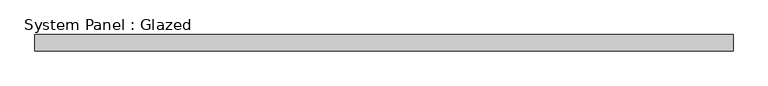
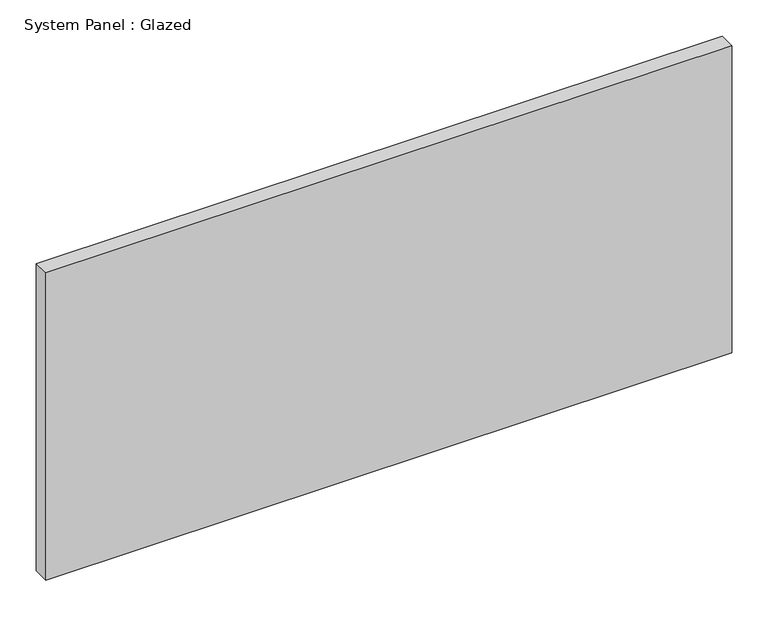
"""IFC4 building model written with IfcOpenShell, lengths in millimetres: plate geometry, System Panel : Glazed."""

from ifc_helpers import new_model, si_unit, origin, origin_with_axes, place, context, project, spatial, polyline, outline, extrude, source, transform, mapped, element, save


def system_panel_glazed_3501c433(model_context):
    return source(origin(), model_context, "Body", "SweptSolid", [
        extrude(outline(polyline([(542.9250001, 19.05), (-542.9250001, 19.05), (-542.9250001, 44.45), (542.9250001, 44.45), (542.9250001, 19.05)])), origin_with_axes(), (0.0, 0.0, 1.0), 514.35),
    ])


if __name__ == "__main__":
    model = new_model("IFC4")
    model_context = context("Model", 3, world=origin())
    ifc_project = project(units=[si_unit("LENGTHUNIT", "METRE", prefix="MILLI")], contexts=[model_context])
    site = spatial("IfcSite", under=ifc_project)
    building = spatial("IfcBuilding", under=site)
    placement = place(None, origin())
    system_panel_glazed_shape = system_panel_glazed_3501c433(model_context)
    element("IfcPlate", 1, ObjectType="System Panel : Glazed", at=placement, inside=building, context=model_context, shape_type="MappedRepresentation", body=[
        mapped(system_panel_glazed_shape, transform((0.0, 0.0, 0.0), x_axis=(1.0, 0.0, 0.0), y_axis=(0.0, 1.0, 0.0), z_axis=(0.0, 0.0, 1.0))),
    ])
    save(model, "model.ifc")

# Revit data of these elements
# Type "System Panel : Glazed"
#   Construction Type Id = "GSP4R"
#   Analytic Construction = "1/8 in Pilkington single glazing"
#   Visual Light Transmittance = 0.9
#   Solar Heat Gain Coefficient = 0.86
#   Heat Transfer Coefficient (U) = 1.18115 BTU/(h·ft²·°F)
#   Define Thermal Properties by = 1
# Element 1 (IfcPlate, "System Panel : Glazed")
#   Materials on its faces: "Glass"
# Materials
#   "Glass": class "Glass", colour RGB 0 128 192, transparency 0.75, Description = "Soda Lime Glass", Cost = 0
